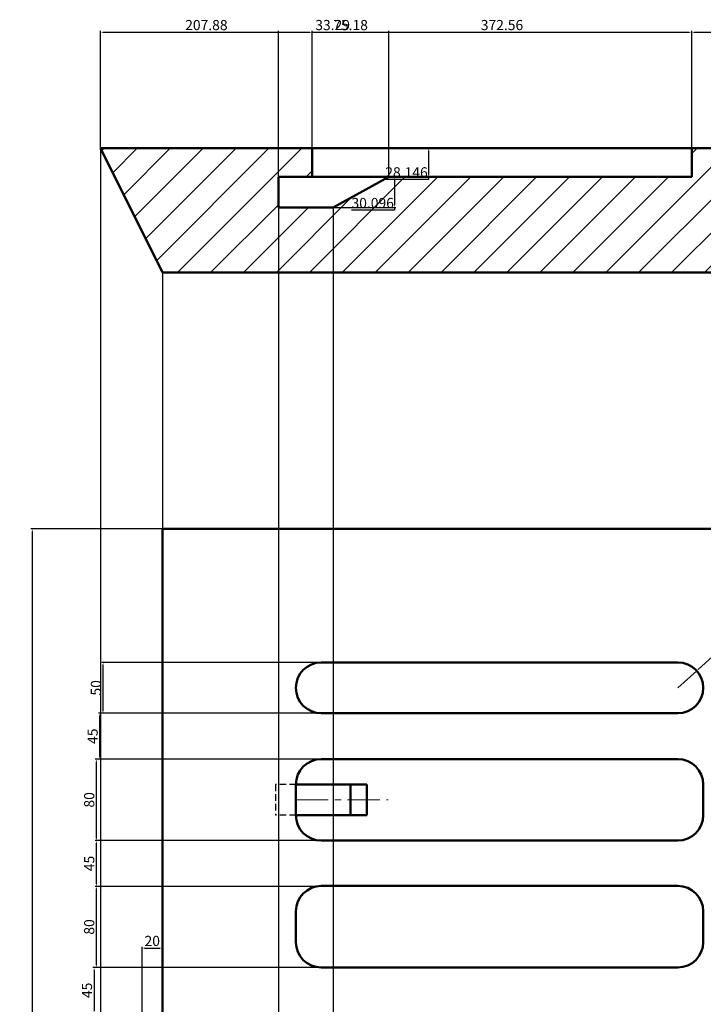
# Model space of a CAD drawing. Units: millimetres. Extents: x 1178 to 3717, y 924 to 2764.
# Tile 4 of 5: x 1799 to 2471, y 1785 to 2752. Entities that reach past the tile are written whole.
import ezdxf

# ---------------------------------------------------------------- set-up
doc = ezdxf.new("R2010")
doc.units = ezdxf.units.MM
doc.linetypes.add('CENTER', pattern=[50.8, 31.75, -6.35, 6.35, -6.35])
doc.linetypes.add('HIDDEN', pattern=[9.525, 6.35, -3.175])
for name, color, linetype, lineweight in [('M-CNTR', 1, 'CENTER', 18), ('M-DIMS', 2, 'Continuous', 25), ('M-HATC', 8, 'Continuous', 18), ('M-HIDN', 6, 'HIDDEN', 25), ('M-OUTL', 7, 'Continuous', 50)]:
    doc.layers.add(name, color=color, linetype=linetype, lineweight=lineweight)
doc.styles.get("Standard").update_dxf_attribs({"font": 'arial.ttf'})
doc.dimstyles.new('ISO-25', dxfattribs={"dimtxt": 10, "dimasz": 2.5, "dimexe": 1.25, "dimexo": 0.625, "dimtad": 1, "dimtoh": 1, "dimdec": 0, "dimtxsty": 'Standard', "dimcen": 2.5, "dimadec": 0, "dimazin": 0, "dimtfac": 1, "dimtdec": 0, "dimtmove": 0, "dimatfit": 3, "dimfxl": 1, "dimarcsym": 0})

# ---------------------------------------------------------------- blocks, each defined once
blk = doc.blocks.new('*D2')
at = {"layer": 'Defpoints', "color": 0, "transparency": 16777216}
for p in [(1939.54, 2252.21), (1811.7, 1051.02), (1939.54, 1051.02)]:
    blk.add_point(p, dxfattribs=at)
at = {"layer": 'M-DIMS', "color": 0, "lineweight": -2, "transparency": 16777216}
for p, q in [((1938.91, 2252.21), (1810.45, 2252.21)), ((1811.7, 2249.71), (1811.7, 1053.52)), ((1938.91, 1051.02), (1810.45, 1051.02))]:
    blk.add_line(p, q, dxfattribs=at)
at = {"layer": 'M-DIMS', "color": 0, "transparency": 16777216}
for points in [[(1811.29, 2249.71), (1812.12, 2249.71), (1811.7, 2252.21)], [(1811.29, 1053.52), (1812.12, 1053.52), (1811.7, 1051.02)]]:
    blk.add_solid(points, dxfattribs=at)
at = {"layer": 'M-DIMS', "color": 0, "transparency": 16777216, "insert": (1805.97, 1651.62), "char_height": 10, "attachment_point": 5, "rotation": 90}
blk.add_mtext('1201', dxfattribs=at)
blk = doc.blocks.new('*D14')
at = {"layer": 'Defpoints', "color": 0, "transparency": 16777216}
for p in [(2095.54, 1821.62), (1872.45, 1776.62), (2095.54, 1776.62)]:
    blk.add_point(p, dxfattribs=at)
at = {"layer": 'M-DIMS', "color": 0, "lineweight": -2, "transparency": 16777216}
for p, q in [((2094.91, 1821.62), (1871.2, 1821.62)), ((1872.45, 1819.12), (1872.45, 1779.12)), ((2094.91, 1776.62), (1871.2, 1776.62))]:
    blk.add_line(p, q, dxfattribs=at)
at = {"layer": 'M-DIMS', "color": 0, "transparency": 16777216}
for points in [[(1872.03, 1819.12), (1872.87, 1819.12), (1872.45, 1821.62)], [(1872.03, 1779.12), (1872.87, 1779.12), (1872.45, 1776.62)]]:
    blk.add_solid(points, dxfattribs=at)
at = {"layer": 'M-DIMS', "color": 0, "transparency": 16777216, "insert": (1866.74, 1799.12), "char_height": 10, "attachment_point": 5, "rotation": 90}
blk.add_mtext('45', dxfattribs=at)
blk = doc.blocks.new('*D16')
at = {"layer": 'Defpoints', "color": 0, "transparency": 16777216}
for p in [(1874.68, 1901.21), (2095.54, 1901.21), (2095.54, 1821.62)]:
    blk.add_point(p, dxfattribs=at)
at = {"layer": 'M-DIMS', "color": 0, "lineweight": -2, "transparency": 16777216}
for p, q in [((2094.91, 1901.21), (1873.43, 1901.21)), ((1874.68, 1824.12), (1874.68, 1898.71)), ((2094.91, 1821.62), (1873.43, 1821.62))]:
    blk.add_line(p, q, dxfattribs=at)
at = {"layer": 'M-DIMS', "color": 0, "transparency": 16777216}
for points in [[(1874.26, 1898.71), (1875.1, 1898.71), (1874.68, 1901.21)], [(1874.26, 1824.12), (1875.1, 1824.12), (1874.68, 1821.62)]]:
    blk.add_solid(points, dxfattribs=at)
at = {"layer": 'M-DIMS', "color": 0, "transparency": 16777216, "insert": (1868.95, 1861.42), "char_height": 10, "attachment_point": 5, "rotation": 90}
blk.add_mtext('80', dxfattribs=at)
blk = doc.blocks.new('*D17')
at = {"layer": 'Defpoints', "color": 0, "transparency": 16777216}
for p in [(1874.68, 1946.21), (2095.54, 1946.21), (2095.54, 1901.21)]:
    blk.add_point(p, dxfattribs=at)
at = {"layer": 'M-DIMS', "color": 0, "lineweight": -2, "transparency": 16777216}
for p, q in [((2094.91, 1946.21), (1873.43, 1946.21)), ((1874.68, 1903.71), (1874.68, 1943.71)), ((2094.91, 1901.21), (1873.43, 1901.21))]:
    blk.add_line(p, q, dxfattribs=at)
at = {"layer": 'M-DIMS', "color": 0, "transparency": 16777216}
for points in [[(1874.26, 1943.71), (1875.1, 1943.71), (1874.68, 1946.21)], [(1874.26, 1903.71), (1875.1, 1903.71), (1874.68, 1901.21)]]:
    blk.add_solid(points, dxfattribs=at)
at = {"layer": 'M-DIMS', "color": 0, "transparency": 16777216, "insert": (1868.97, 1923.71), "char_height": 10, "attachment_point": 5, "rotation": 90}
blk.add_mtext('45', dxfattribs=at)
blk = doc.blocks.new('*D18')
at = {"layer": 'Defpoints', "color": 0, "transparency": 16777216}
for p in [(1874.68, 2026.21), (2095.54, 2026.21), (2095.54, 1946.21)]:
    blk.add_point(p, dxfattribs=at)
at = {"layer": 'M-DIMS', "color": 0, "lineweight": -2, "transparency": 16777216}
for p, q in [((2094.91, 2026.21), (1873.43, 2026.21)), ((1874.68, 1948.71), (1874.68, 2023.71)), ((2094.91, 1946.21), (1873.43, 1946.21))]:
    blk.add_line(p, q, dxfattribs=at)
at = {"layer": 'M-DIMS', "color": 0, "transparency": 16777216}
for points in [[(1874.26, 2023.71), (1875.1, 2023.71), (1874.68, 2026.21)], [(1874.26, 1948.71), (1875.1, 1948.71), (1874.68, 1946.21)]]:
    blk.add_solid(points, dxfattribs=at)
at = {"layer": 'M-DIMS', "color": 0, "transparency": 16777216, "insert": (1868.95, 1986.21), "char_height": 10, "attachment_point": 5, "rotation": 90}
blk.add_mtext('80', dxfattribs=at)
blk = doc.blocks.new('*D19')
at = {"layer": 'Defpoints', "color": 0, "transparency": 16777216}
for p in [(1877.99, 2071.21), (2095.54, 2071.21), (2095.54, 2026.21)]:
    blk.add_point(p, dxfattribs=at)
at = {"layer": 'M-DIMS', "color": 0, "lineweight": -2, "transparency": 16777216}
for p, q in [((2094.91, 2071.21), (1876.74, 2071.21)), ((1877.99, 2028.71), (1877.99, 2068.71)), ((2094.91, 2026.21), (1876.74, 2026.21))]:
    blk.add_line(p, q, dxfattribs=at)
at = {"layer": 'M-DIMS', "color": 0, "transparency": 16777216}
for points in [[(1877.58, 2068.71), (1878.41, 2068.71), (1877.99, 2071.21)], [(1877.58, 2028.71), (1878.41, 2028.71), (1877.99, 2026.21)]]:
    blk.add_solid(points, dxfattribs=at)
at = {"layer": 'M-DIMS', "color": 0, "transparency": 16777216, "insert": (1872.28, 2048.71), "char_height": 10, "attachment_point": 5, "rotation": 90}
blk.add_mtext('45', dxfattribs=at)
blk = doc.blocks.new('*D20')
at = {"layer": 'Defpoints', "color": 0, "transparency": 16777216}
for p in [(1881.27, 2121.21), (2095.54, 2121.21), (2095.54, 2071.21)]:
    blk.add_point(p, dxfattribs=at)
at = {"layer": 'M-DIMS', "color": 0, "lineweight": -2, "transparency": 16777216}
for p, q in [((2094.91, 2121.21), (1880.02, 2121.21)), ((1881.27, 2073.71), (1881.27, 2118.71)), ((2094.91, 2071.21), (1880.02, 2071.21))]:
    blk.add_line(p, q, dxfattribs=at)
at = {"layer": 'M-DIMS', "color": 0, "transparency": 16777216}
for points in [[(1880.85, 2118.71), (1881.68, 2118.71), (1881.27, 2121.21)], [(1880.85, 2073.71), (1881.68, 2073.71), (1881.27, 2071.21)]]:
    blk.add_solid(points, dxfattribs=at)
at = {"layer": 'M-DIMS', "color": 0, "transparency": 16777216, "insert": (1875.53, 2096.21), "char_height": 10, "attachment_point": 5, "rotation": 90}
blk.add_mtext('50', dxfattribs=at)
blk = doc.blocks.new('*D23')
at = {"layer": 'Defpoints', "color": 0, "transparency": 16777216}
for p in [(2464.1, 2112.97), (2445.54, 2096.21)]:
    blk.add_point(p, dxfattribs=at)
at = {"layer": 'M-DIMS', "color": 0, "lineweight": -2, "transparency": 16777216}
for p, q in [((2681.27, 2309.04), (2465.95, 2114.64)), ((2705.86, 2309.04), (2681.27, 2309.04)), ((2445.54, 2096.21), (2464.1, 2112.97))]:
    blk.add_line(p, q, dxfattribs=at)
at = {"layer": 'M-DIMS', "color": 0, "transparency": 16777216}
blk.add_solid([(2465.67, 2114.95), (2466.23, 2114.33), (2464.1, 2112.97)], dxfattribs=at)
at = {"layer": 'M-DIMS', "color": 0, "transparency": 16777216, "insert": (2693.88, 2314.77), "char_height": 10, "attachment_point": 5}
blk.add_mtext('R25', dxfattribs=at)
blk = doc.blocks.new('SLOT-400X50')
for p, q in [((375, 50), (25, 50)), ((25, 0), (375, 0))]:
    blk.add_line(p, q)
for centre, start, end in [((25, 25), 90, 270), ((375, 25), 270, 90)]:
    blk.add_arc(centre, 25, start, end)
blk = doc.blocks.new('*D28')
at = {"layer": 'Defpoints', "color": 0, "transparency": 16777216}
for p in [(1878.75, 2626.04), (1939.54, 2504.04), (1939.54, 937.02)]:
    blk.add_point(p, dxfattribs=at)
at = {"layer": 'M-DIMS', "color": 0, "lineweight": -2, "transparency": 16777216}
for p, q in [((1878.75, 2625.42), (1878.75, 935.77)), ((1939.54, 2503.42), (1939.54, 935.77)), ((1881.25, 937.02), (1937.04, 937.02))]:
    blk.add_line(p, q, dxfattribs=at)
at = {"layer": 'M-DIMS', "color": 0, "transparency": 16777216}
for points in [[(1881.25, 937.44), (1881.25, 936.61), (1878.75, 937.02)], [(1937.04, 937.44), (1937.04, 936.61), (1939.54, 937.02)]]:
    blk.add_solid(points, dxfattribs=at)
at = {"layer": 'M-DIMS', "color": 0, "transparency": 16777216, "insert": (1909.15, 942.75), "char_height": 10, "attachment_point": 5}
blk.add_mtext('60.79', dxfattribs=at)
blk = doc.blocks.new('*D29')
at = {"layer": 'Defpoints', "color": 0, "transparency": 16777216}
for p in [(2086.63, 2740.04), (1878.75, 2626.04), (2086.63, 2626.04)]:
    blk.add_point(p, dxfattribs=at)
at = {"layer": 'M-DIMS', "color": 0, "lineweight": -2, "transparency": 16777216}
for p, q in [((1878.75, 2626.67), (1878.75, 2741.29)), ((1881.25, 2740.04), (2084.13, 2740.04)), ((2086.63, 2626.67), (2086.63, 2741.29))]:
    blk.add_line(p, q, dxfattribs=at)
at = {"layer": 'M-DIMS', "color": 0, "transparency": 16777216}
for points in [[(1881.25, 2740.46), (1881.25, 2739.62), (1878.75, 2740.04)], [(2084.13, 2740.46), (2084.13, 2739.62), (2086.63, 2740.04)]]:
    blk.add_solid(points, dxfattribs=at)
at = {"layer": 'M-DIMS', "color": 0, "transparency": 16777216, "insert": (1982.69, 2745.77), "char_height": 10, "attachment_point": 5}
blk.add_mtext('207.88', dxfattribs=at)
blk = doc.blocks.new('*D30')
at = {"layer": 'Defpoints', "color": 0, "transparency": 16777216}
for p in [(2459.19, 2740.04), (2086.63, 2626.04), (2459.19, 2626.04)]:
    blk.add_point(p, dxfattribs=at)
at = {"layer": 'M-DIMS', "color": 0, "lineweight": -2, "transparency": 16777216}
for p, q in [((2086.63, 2626.67), (2086.63, 2741.29)), ((2089.13, 2740.04), (2456.69, 2740.04)), ((2459.19, 2626.67), (2459.19, 2741.29))]:
    blk.add_line(p, q, dxfattribs=at)
at = {"layer": 'M-DIMS', "color": 0, "transparency": 16777216}
for points in [[(2089.13, 2740.46), (2089.13, 2739.62), (2086.63, 2740.04)], [(2456.69, 2740.46), (2456.69, 2739.62), (2459.19, 2740.04)]]:
    blk.add_solid(points, dxfattribs=at)
at = {"layer": 'M-DIMS', "color": 0, "transparency": 16777216, "insert": (2272.91, 2745.78), "char_height": 10, "attachment_point": 5}
blk.add_mtext('372.56', dxfattribs=at)
blk = doc.blocks.new('*D31')
at = {"layer": 'Defpoints', "color": 0, "transparency": 16777216}
for p in [(2565.41, 2740.04), (2459.19, 2626.04), (2565.41, 2626.04)]:
    blk.add_point(p, dxfattribs=at)
at = {"layer": 'M-DIMS', "color": 0, "lineweight": -2, "transparency": 16777216}
for p, q in [((2459.19, 2626.67), (2459.19, 2741.29)), ((2461.69, 2740.04), (2562.91, 2740.04)), ((2565.41, 2626.67), (2565.41, 2741.29))]:
    blk.add_line(p, q, dxfattribs=at)
at = {"layer": 'M-DIMS', "color": 0, "transparency": 16777216}
for points in [[(2461.69, 2740.46), (2461.69, 2739.62), (2459.19, 2740.04)], [(2562.91, 2740.46), (2562.91, 2739.62), (2565.41, 2740.04)]]:
    blk.add_solid(points, dxfattribs=at)
at = {"layer": 'M-DIMS', "color": 0, "transparency": 16777216, "insert": (2512.3, 2745.77), "char_height": 10, "attachment_point": 5}
blk.add_mtext('106.22', dxfattribs=at)
blk = doc.blocks.new('*D39')
at = {"layer": 'Defpoints', "color": 0, "transparency": 16777216}
for p in [(2086.63, 2626.04), (2086.63, 2597.9), (2200.63, 2597.9)]:
    blk.add_point(p, dxfattribs=at)
at = {"layer": 'M-DIMS', "color": 0, "lineweight": -2, "transparency": 16777216}
for p, q in [((2087.25, 2626.04), (2201.88, 2626.04)), ((2200.63, 2623.54), (2200.63, 2600.4)), ((2087.25, 2597.9), (2201.88, 2597.9)), ((2200.63, 2595.4), (2158.33, 2595.4)), ((2200.63, 2597.9), (2200.63, 2595.4))]:
    blk.add_line(p, q, dxfattribs=at)
at = {"layer": 'M-DIMS', "color": 0, "transparency": 16777216}
for points in [[(2200.21, 2623.54), (2201.05, 2623.54), (2200.63, 2626.04)], [(2200.21, 2600.4), (2201.05, 2600.4), (2200.63, 2597.9)]]:
    blk.add_solid(points, dxfattribs=at)
at = {"layer": 'M-DIMS', "color": 0, "transparency": 16777216, "insert": (2179.17, 2601.13), "char_height": 10, "attachment_point": 5}
blk.add_mtext('28.146', dxfattribs=at)
blk = doc.blocks.new('*D40')
at = {"layer": 'Defpoints', "color": 0, "transparency": 16777216}
for p in [(2053.34, 2597.9), (2053.34, 2567.8), (2167.34, 2567.8)]:
    blk.add_point(p, dxfattribs=at)
at = {"layer": 'M-DIMS', "color": 0, "lineweight": -2, "transparency": 16777216}
for p, q in [((2053.96, 2597.9), (2168.59, 2597.9)), ((2167.34, 2595.4), (2167.34, 2570.3)), ((2053.96, 2567.8), (2168.59, 2567.8)), ((2167.34, 2565.3), (2125.21, 2565.3)), ((2167.34, 2567.8), (2167.34, 2565.3))]:
    blk.add_line(p, q, dxfattribs=at)
at = {"layer": 'M-DIMS', "color": 0, "transparency": 16777216}
for points in [[(2166.92, 2595.4), (2167.75, 2595.4), (2167.34, 2597.9)], [(2166.92, 2570.3), (2167.75, 2570.3), (2167.34, 2567.8)]]:
    blk.add_solid(points, dxfattribs=at)
at = {"layer": 'M-DIMS', "color": 0, "transparency": 16777216, "insert": (2145.96, 2571.03), "char_height": 10, "attachment_point": 5}
blk.add_mtext('30.096', dxfattribs=at)
blk = doc.blocks.new('*D41')
at = {"layer": 'Defpoints', "color": 0, "transparency": 16777216}
for p in [(2086.63, 2740.04), (2053.34, 2597.9), (2086.63, 2597.9)]:
    blk.add_point(p, dxfattribs=at)
at = {"layer": 'M-DIMS', "color": 0, "lineweight": -2, "transparency": 16777216}
for p, q in [((2053.34, 2598.52), (2053.34, 2741.29)), ((2055.84, 2740.04), (2084.13, 2740.04)), ((2086.63, 2598.52), (2086.63, 2741.29)), ((2086.63, 2740.04), (2124.14, 2740.04))]:
    blk.add_line(p, q, dxfattribs=at)
at = {"layer": 'M-DIMS', "color": 0, "transparency": 16777216}
for points in [[(2055.84, 2740.46), (2055.84, 2739.62), (2053.34, 2740.04)], [(2084.13, 2740.46), (2084.13, 2739.62), (2086.63, 2740.04)]]:
    blk.add_solid(points, dxfattribs=at)
at = {"layer": 'M-DIMS', "color": 0, "transparency": 16777216, "insert": (2106.63, 2745.78), "char_height": 10, "attachment_point": 5}
blk.add_mtext('33.29', dxfattribs=at)
blk = doc.blocks.new('*D42')
at = {"layer": 'Defpoints', "color": 0, "transparency": 16777216}
for p in [(2161.81, 2740.04), (2086.63, 2597.9), (2161.81, 2597.9)]:
    blk.add_point(p, dxfattribs=at)
at = {"layer": 'M-DIMS', "color": 0, "lineweight": -2, "transparency": 16777216}
for p, q in [((2086.63, 2598.52), (2086.63, 2741.29)), ((2089.13, 2740.04), (2159.31, 2740.04)), ((2161.81, 2598.52), (2161.81, 2741.29))]:
    blk.add_line(p, q, dxfattribs=at)
at = {"layer": 'M-DIMS', "color": 0, "transparency": 16777216}
for points in [[(2089.13, 2740.46), (2089.13, 2739.62), (2086.63, 2740.04)], [(2159.31, 2740.46), (2159.31, 2739.62), (2161.81, 2740.04)]]:
    blk.add_solid(points, dxfattribs=at)
at = {"layer": 'M-DIMS', "color": 0, "transparency": 16777216, "insert": (2124.22, 2745.77), "char_height": 10, "attachment_point": 5}
blk.add_mtext('75.18', dxfattribs=at)
blk = doc.blocks.new('*D43')
at = {"layer": 'Defpoints', "color": 0, "transparency": 16777216}
for p in [(2053.34, 2567.8), (2107.24, 2567.8), (2107.24, 937.02)]:
    blk.add_point(p, dxfattribs=at)
at = {"layer": 'M-DIMS', "color": 0, "lineweight": -2, "transparency": 16777216}
for p, q in [((2053.34, 2567.18), (2053.34, 935.77)), ((2107.24, 2567.18), (2107.24, 935.77)), ((2055.84, 937.02), (2104.74, 937.02))]:
    blk.add_line(p, q, dxfattribs=at)
at = {"layer": 'M-DIMS', "color": 0, "transparency": 16777216}
for points in [[(2055.84, 937.44), (2055.84, 936.61), (2053.34, 937.02)], [(2104.74, 937.44), (2104.74, 936.61), (2107.24, 937.02)]]:
    blk.add_solid(points, dxfattribs=at)
at = {"layer": 'M-DIMS', "color": 0, "transparency": 16777216, "insert": (2080.29, 942.76), "char_height": 10, "attachment_point": 5}
blk.add_mtext('53.9', dxfattribs=at)
blk = doc.blocks.new('*D55')
at = {"layer": 'Defpoints', "color": 0, "transparency": 16777216}
for p in [(1939.54, 1840.62), (1919.54, 1726.62), (1939.54, 1726.62)]:
    blk.add_point(p, dxfattribs=at)
at = {"layer": 'M-DIMS', "color": 0, "lineweight": -2, "transparency": 16777216}
for p, q in [((1919.54, 1727.24), (1919.54, 1841.87)), ((1922.04, 1840.62), (1937.04, 1840.62)), ((1939.54, 1727.24), (1939.54, 1841.87))]:
    blk.add_line(p, q, dxfattribs=at)
at = {"layer": 'M-DIMS', "color": 0, "transparency": 16777216}
for points in [[(1922.04, 1841.03), (1922.04, 1840.2), (1919.54, 1840.62)], [(1937.04, 1841.03), (1937.04, 1840.2), (1939.54, 1840.62)]]:
    blk.add_solid(points, dxfattribs=at)
at = {"layer": 'M-DIMS', "color": 0, "transparency": 16777216, "insert": (1929.54, 1846.35), "char_height": 10, "attachment_point": 5}
blk.add_mtext('20', dxfattribs=at)

msp = doc.modelspace()

# ---------------------------------------------------------------- hatches: boundary and pattern name
at = {"layer": 'M-HATC'}
h = msp.add_hatch(dxfattribs=at)
h.set_pattern_fill('ANSI31', color=256, scale=7.2)
h.paths.add_polyline_path([(2053.3369, 2597.896), (2086.6296, 2597.896), (2086.6296, 2626.0416), (1939.5398, 2626.0416), (1878.7536, 2626.0416), (1939.5398, 2504.0416), (2764.9597, 2504.0416), (2764.9597, 2589.9761), (2565.4108, 2589.9761), (2565.4108, 2626.0416), (2459.1911, 2626.0416), (2459.1911, 2597.896), (2161.8062, 2597.896), (2107.2394, 2567.8003), (2053.3369, 2567.8003)])
h.paths.add_polyline_path([(3590.3795, 2626.0416), (3397.729, 2626.0416), (3397.729, 2585.2241), (3441.1717, 2585.2241), (3441.1717, 2561.8005), (3373.4902, 2561.8005), (3343.1801, 2585.2241), (2990.2894, 2585.2241), (2990.2894, 2626.0416), (2880.899, 2626.0416), (2880.899, 2589.9761), (2764.9597, 2589.9761), (2764.9597, 2504.0416), (3521.5398, 2504.0416)])

# ---------------------------------------------------------------- linework, layer by layer
at = {"layer": 'M-CNTR'}
msp.add_line((2070.5398, 1986.2134), (2161.1852, 1986.2134), dxfattribs=at)
at = {"layer": 'M-HIDN'}
for p, q in [((2070.5398, 2001.2134), (2050.6046, 2001.2134)), ((2050.6046, 2001.2134), (2050.6046, 1971.2134)), ((2070.5398, 1971.2134), (2050.6046, 1971.2134))]:
    msp.add_line(p, q, dxfattribs=at)
at = {"layer": 'M-OUTL'}
for p, q in [((1939.5398, 2626.0416), (1878.7536, 2626.0416)), ((1878.7536, 2626.0416), (1939.5398, 2504.0416)), ((1939.5398, 2626.0416), (3590.3795, 2626.0416)), ((2086.6296, 2626.0416), (2086.6296, 2597.896)), ((2459.1911, 2597.896), (2459.1911, 2626.0416)), ((2086.6296, 2597.896), (2053.3369, 2597.896)), ((2053.3369, 2597.896), (2053.3369, 2567.8003)), ((2086.6296, 2597.896), (2459.1911, 2597.896)), ((2107.2394, 2567.8003), (2161.8062, 2597.896)), ((2053.3369, 2567.8003), (2107.2394, 2567.8003)), ((3521.5398, 2504.0416), (1939.5398, 2504.0416)), ((2095.5398, 2252.2134), (1939.5398, 2252.2134)), ((1939.5398, 1903.0224), (1939.5398, 2252.2134)), ((2095.5398, 2252.2134), (3521.5398, 2252.2134)), ((2095.5398, 2026.2134), (2445.5398, 2026.2134)), ((2070.5398, 1971.2134), (2070.5398, 2001.2134)), ((2070.5398, 1971.2134), (2070.5398, 2001.2134)), ((2070.5398, 2001.2134), (2140.3627, 2001.2134)), ((2124.325, 1971.2134), (2124.325, 2001.2134)), ((2140.3627, 2001.2134), (2140.3627, 1971.2134)), ((2470.5398, 2001.2134), (2470.5398, 1971.2134)), ((2070.5398, 1971.2134), (2140.3627, 1971.2134)), ((2445.5398, 1946.2134), (2095.5398, 1946.2134)), ((1939.5398, 1903.0224), (1939.5398, 1726.6179)), ((2095.5398, 1901.6179), (2095.5398, 1901.2134)), ((2095.5398, 1901.6179), (2445.5398, 1901.6179)), ((2070.5398, 1846.6179), (2070.5398, 1876.6179)), ((2470.5398, 1876.6179), (2470.5398, 1846.6179)), ((2445.5398, 1821.6179), (2095.5398, 1821.6179))]:
    msp.add_line(p, q, dxfattribs=at)
for centre, start, end in [((2095.5398, 2001.2134), 90, 180), ((2445.5398, 2001.2134), 0, 90), ((2095.5398, 1971.2134), 180, 270), ((2445.5398, 1971.2134), 270, 0), ((2095.5398, 1876.6179), 90, 180), ((2445.5398, 1876.6179), 0, 90), ((2095.5398, 1846.6179), 180, 270), ((2445.5398, 1846.6179), 270, 0)]:
    msp.add_arc(centre, 25, start, end, dxfattribs=at)

# ---------------------------------------------------------------- block references
msp.add_blockref('SLOT-400X50', (2070.54, 2071.213), dxfattribs=at)

# ---------------------------------------------------------------- dimensions: what is measured, and where the dimension line sits
at = {"layer": 'M-DIMS'}
for base, p1, p2, override, picture, middle in [((2086.6296, 2740.0416), (1878.7536, 2626.0416), (2086.6296, 2626.0416), {"dimdec": 2, "dimlfac": 1, "dimrnd": 0, "dimzin": 0, "dimdsep": 46, "dimlunit": 2}, '*D29', (1982.6916, 2745.7723)), ((2086.6296, 2740.0416), (2053.3369, 2597.896), (2086.6296, 2597.896), {"dimdec": 2, "dimlfac": 1, "dimrnd": 0, "dimzin": 0, "dimdsep": 46, "dimlunit": 2}, '*D41', (2106.6339, 2745.7757)), ((2459.1911, 2740.0416), (2086.6296, 2626.0416), (2459.1911, 2626.0416), {"dimdec": 2, "dimlfac": 1, "dimrnd": 0, "dimzin": 0, "dimdsep": 46, "dimlunit": 2}, '*D30', (2272.9104, 2745.7757)), ((2161.8062, 2740.0416), (2086.6296, 2597.896), (2161.8062, 2597.896), {"dimdec": 2, "dimlfac": 1, "dimrnd": 0, "dimzin": 0, "dimdsep": 46, "dimlunit": 2}, '*D42', (2124.2179, 2745.7723)), ((2565.4108, 2740.0416), (2459.1911, 2626.0416), (2565.4108, 2626.0416), {"dimdec": 2, "dimlfac": 1, "dimrnd": 0, "dimzin": 0, "dimdsep": 46, "dimlunit": 2}, '*D31', (2512.3009, 2745.7723)), ((1939.5398, 937.0224), (1878.7536, 2626.0416), (1939.5398, 2504.0416), {"dimdec": 2, "dimlfac": 1, "dimrnd": 0, "dimzin": 0, "dimdsep": 46, "dimlunit": 2}, '*D28', (1909.1467, 942.7532)), ((2107.2394, 937.0224), (2053.3369, 2567.8003), (2107.2394, 2567.8003), {"dimdec": 1, "dimlfac": 1, "dimrnd": 0, "dimzin": 0, "dimdsep": 46, "dimlunit": 2}, '*D43', (2080.2882, 942.7566)), ((1939.5398, 1840.6179), (1919.5398, 1726.6179), (1939.5398, 1726.6179), {"dimdec": 0, "dimlfac": 1, "dimrnd": 0, "dimzin": 0, "dimdsep": 46, "dimlunit": 2}, '*D55', (1929.5398, 1846.3487))]:
    dim = msp.add_linear_dim(base=base, p1=p1, p2=p2, dimstyle='ISO-25', override=override, dxfattribs=at)
    dim.commit()
    dim.dimension.update_dxf_attribs({"geometry": picture, "text_midpoint": middle})
for base, p1, p2, angle, override, picture, middle in [((2200.6296, 2597.896), (2086.6296, 2626.0416), (2086.6296, 2597.896), 270, {"dimdec": 3, "dimlfac": 1, "dimrnd": 0, "dimzin": 0, "dimdsep": 46, "dimlunit": 2}, '*D39', (2179.1656, 2601.1267)), ((2167.3369, 2567.8003), (2053.3369, 2597.896), (2053.3369, 2567.8003), 270, {"dimdec": 3, "dimlfac": 1, "dimrnd": 0, "dimzin": 0, "dimdsep": 46, "dimlunit": 2}, '*D40', (2145.9616, 2571.0345)), ((1811.7032, 1051.0224), (1939.5398, 2252.2134), (1939.5398, 1051.0224), 90, {"dimclrd": 0, "dimclre": 0, "dimclrt": 0}, '*D2', (1805.9725, 1651.6179)), ((1881.2655, 2121.2134), (2095.5398, 2071.2134), (2095.5398, 2121.2134), 90, {"dimclrd": 0, "dimclre": 0, "dimclrt": 0}, '*D20', (1875.5348, 2096.2134)), ((1877.9926, 2071.2134), (2095.5398, 2026.2134), (2095.5398, 2071.2134), 90, {"dimclrd": 0, "dimclre": 0, "dimclrt": 0}, '*D19', (1872.2823, 2048.7134)), ((1874.6801, 2026.2134), (2095.5398, 1946.2134), (2095.5398, 2026.2134), 90, {"dimclrd": 0, "dimclre": 0, "dimclrt": 0}, '*D18', (1868.9494, 1986.2134)), ((1874.6801, 1946.2134), (2095.5398, 1901.2134), (2095.5398, 1946.2134), 90, {"dimclrd": 0, "dimclre": 0, "dimclrt": 0}, '*D17', (1868.9698, 1923.7134)), ((1874.6801, 1901.2134), (2095.5398, 1821.6179), (2095.5398, 1901.2134), 90, {"dimclrd": 0, "dimclre": 0, "dimclrt": 0}, '*D16', (1868.9494, 1861.4157)), ((1872.4506, 1776.6179), (2095.5398, 1821.6179), (2095.5398, 1776.6179), 90, {"dimclrd": 0, "dimclre": 0, "dimclrt": 0}, '*D14', (1866.7404, 1799.1179))]:
    dim = msp.add_linear_dim(base=base, p1=p1, p2=p2, angle=angle, dimstyle='ISO-25', override=override, dxfattribs=at)
    dim.commit()
    dim.dimension.update_dxf_attribs({"geometry": picture, "text_midpoint": middle})
dim = msp.add_radius_dim(center=(2445.5398, 2096.2134), mpoint=(2464.0957, 2112.9669), dimstyle='ISO-25', override={"dimclrd": 0, "dimclre": 0, "dimclrt": 0}, dxfattribs=at)
dim.commit()
dim.dimension.update_dxf_attribs({"geometry": '*D23', "text_midpoint": (2693.8758, 2309.0425), "dimtype": 164})

doc.saveas('drawing.dxf')
